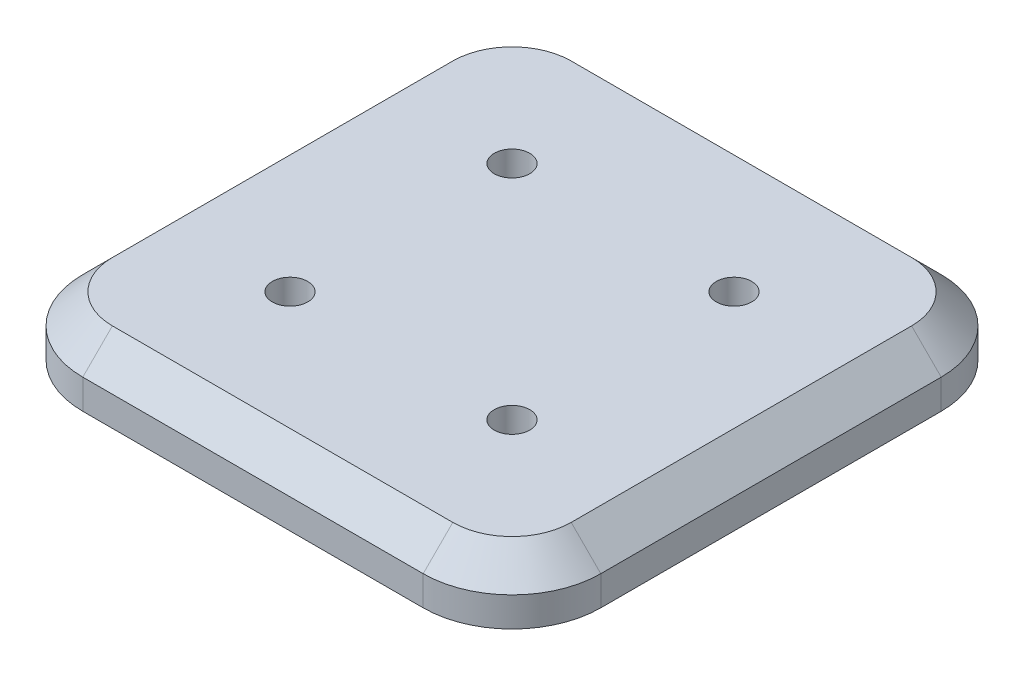
SolidWorks part; units mm, degrees
material "Plain Carbon Steel"
ref_plane "Front Plane" through (0, 0, 0) normal (0, 0, 1) x (1, 0, 0)
ref_plane "Top Plane" through (0, 0, 0) normal (0, 1, 0) x (1, 0, 0)
ref_plane "Right Plane" through (0, 0, 0) normal (1, 0, 0) x (0, 0, -1)
sketch "Base Plate Sketch 175x175" plane through (0, 0, 0) normal (0, 1, 0) x (1, 0, 0)
  line L1 (-87.5, -87.5) -> (87.5, -87.5)
  line L2 (-87.5, -87.5) -> (-87.5, 87.5)
  line L3 (-87.5, 87.5) -> (87.5, 87.5)
  line L4 (87.5, -87.5) -> (87.5, 87.5)
  line L5 (-87.5, -87.5) -> (87.5, 87.5) construction
  line L6 (-87.5, 87.5) -> (87.5, -87.5) construction
  point P0 (0, 0)
  dimension "D1" = 175
  dimension "D2" = 175
extrude "Base Plate" add sketch "Base Plate Sketch 175x175" along normal blind 20
fillet "Corner Fillets R30" radius 30 4 edges at (-87.5, 10, -87.5) (87.5, 10, -87.5) (87.5, 10, 87.5) (-87.5, 10, 87.5)
chamfer "Edge Chamfer 10x45" distance 10 angle 45 8 edges at (0, 20, -87.5) (-78.7132, 20, -78.7132) (78.7132, 20, -78.7132) (-87.5, 20, 0) (87.5, 20, 0) (-78.7132, 20, 78.7132) (78.7132, 20, 78.7132) (0, 20, 87.5)
sketch "Inner Dowel Layout 75x75" plane through (0, 20, 0) normal (0, 1, 0) x (1, 0, 0)
  line L1 (-37.5, -37.5) -> (37.5, -37.5)
  line L2 (-37.5, -37.5) -> (-37.5, 37.5)
  line L3 (-37.5, 37.5) -> (37.5, 37.5)
  line L4 (37.5, -37.5) -> (37.5, 37.5)
  line L5 (-37.5, -37.5) -> (37.5, 37.5) construction
  line L6 (-37.5, 37.5) -> (37.5, -37.5) construction
  point P0 (0, 0)
  dimension "D1" = 75
  dimension "D2" = 75
hole_wizard "Dowel Holes Ø12 Inner" positions "3DSketch1" profile "Sketch3" hole size "Ø12.0" standard "ANSI Metric"
sketch3d "3DSketch1"
  point P0 (-37.5, 20, -37.5)
  point P3 (37.5, 20, -37.5)
  point P6 (37.5, 20, 37.5)
  point P9 (-37.5, 20, 37.5)
sketch "Sketch3" plane through (-37.5, 20, -37.5) normal (1, 0, 0) x (0, 0, 1)
  line L0 (0, 0) -> (0, 13.6052)
  line L1 (0, 13.6052) -> (6, 10)
  line L2 (6, 10) -> (6, 0)
  line L5 (6, 0) -> (0, 0)
  line L10 (0, 13.6052) -> (-6, 10) construction
  line L11 (0, -6.35) -> (0, 107.95) construction
  dimension "Hole Dia." = 12
  dimension "Hole Depth" = 10
  dimension "Drill Angle" = 118
sketch "Outer Dowel Layout 125x125" plane through (0, 0, 0) normal (0, -1, 0) x (1, 0, 0)
  line L1 (-62.5, -62.5) -> (62.5, -62.5)
  line L2 (-62.5, -62.5) -> (-62.5, 62.5)
  line L3 (-62.5, 62.5) -> (62.5, 62.5)
  line L4 (62.5, -62.5) -> (62.5, 62.5)
  line L5 (-62.5, -62.5) -> (62.5, 62.5) construction
  line L6 (-62.5, 62.5) -> (62.5, -62.5) construction
  point P0 (0, 0)
  dimension "D1" = 125
  dimension "D2" = 125
hole_wizard "Dowel Holes Ø12 Outer" positions "3DSketch2" profile "Sketch5" hole size "Ø12.0" standard "ANSI Metric"
sketch3d "3DSketch2"
  point P0 (-62.5, 0, 62.5)
  point P3 (62.5, 0, 62.5)
  point P6 (62.5, 0, -62.5)
  point P9 (-62.5, 0, -62.5)
sketch "Sketch5" plane through (-62.5, 0, 62.5) normal (1, 0, 0) x (0, 0, -1)
  line L0 (0, 0) -> (0, 13.6052)
  line L1 (0, 13.6052) -> (6, 10)
  line L2 (6, 10) -> (6, 0)
  line L5 (6, 0) -> (0, 0)
  line L10 (0, 13.6052) -> (-6, 10) construction
  line L11 (0, -6.35) -> (0, 107.95) construction
  dimension "Hole Dia." = 12
  dimension "Hole Depth" = 10
  dimension "Drill Angle" = 118
